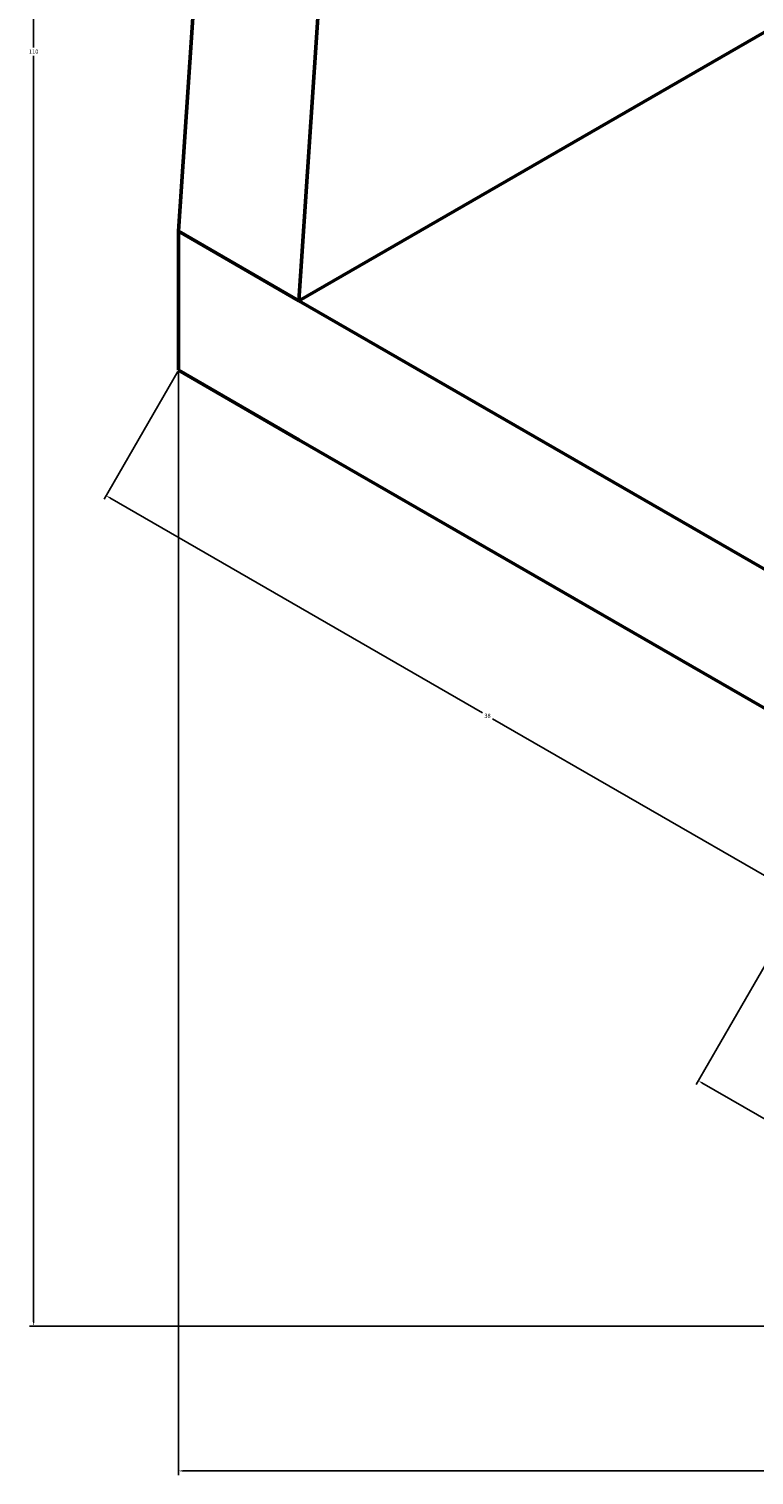
# Model space of a CAD drawing. Units: inches. Extents: x -23 to 69, y -27 to 96.
# Tile 1 of 10: x -23 to 8, y -27 to 35. Entities that reach past the tile are written whole.
import ezdxf

# ---------------------------------------------------------------- set-up
doc = ezdxf.new("R2010")
doc.units = ezdxf.units.IN
doc.header["$MEASUREMENT"] = 0
doc.layers.add('M-DIMS', color=2, linetype='Continuous', lineweight=18)
doc.layers.add('M-OUTL', color=7, linetype='Continuous', lineweight=50)
doc.styles.get("Standard").update_dxf_attribs({"font": 'arial.ttf'})
doc.dimstyles.get("Standard").update_dxf_attribs({"dimtxt": 0.18, "dimasz": 0.18, "dimexe": 0.18, "dimexo": 0.0625, "dimgap": 0.09, "dimtad": 0, "dimtih": 1, "dimtoh": 1, "dimdec": 4, "dimzin": 0, "dimdsep": 46, "dimtxsty": 'Standard', "dimcen": 0.09, "dimadec": 0, "dimazin": 0, "dimtfac": 1, "dimtdec": 4, "dimtofl": 0, "dimtmove": 0, "dimatfit": 3, "dimfxl": 1, "dimtolj": 1, "dimtzin": 0, "dimarcsym": 0})

# ---------------------------------------------------------------- blocks, each defined once
blk = doc.blocks.new('*D2')
at = {"layer": 'Defpoints', "color": 0, "transparency": 16777216}
for p in [(-16.638, 20.369), (-19.763, 14.956), (16.271, 1.369)]:
    blk.add_point(p, dxfattribs=at)
at = {"layer": 'M-DIMS', "color": 0, "lineweight": -2, "transparency": 16777216}
for p, q in [((-16.669, 20.315), (-19.853, 14.8)), ((-19.607, 14.866), (-3.527, 5.582)), ((12.99, -3.954), (-3.089, 5.33)), ((16.24, 1.315), (13.056, -4.2))]:
    blk.add_line(p, q, dxfattribs=at)
at = {"layer": 'M-DIMS', "color": 0, "transparency": 16777216}
for points in [[(-19.592, 14.892), (-19.622, 14.84), (-19.763, 14.956)], [(13.005, -3.928), (12.975, -3.98), (13.146, -4.044)]]:
    blk.add_solid(points, dxfattribs=at)
at = {"layer": 'M-DIMS', "color": 0, "transparency": 16777216, "insert": (-3.308, 5.456), "char_height": 0.18, "attachment_point": 5}
blk.add_mtext('\\A1;38', dxfattribs=at)
blk = doc.blocks.new('*D6')
at = {"layer": 'Defpoints', "color": 0, "transparency": 16777216}
for p in [(8.91, -4.881), (5.785, -10.294), (36.623, -20.881)]:
    blk.add_point(p, dxfattribs=at)
at = {"layer": 'M-DIMS', "color": 0, "lineweight": -2, "transparency": 16777216}
for p, q in [((8.879, -4.935), (5.695, -10.45)), ((5.941, -10.384), (19.423, -18.168)), ((33.342, -26.204), (19.859, -18.42)), ((36.592, -20.935), (33.408, -26.45))]:
    blk.add_line(p, q, dxfattribs=at)
at = {"layer": 'M-DIMS', "color": 0, "transparency": 16777216}
for points in [[(5.956, -10.358), (5.926, -10.41), (5.785, -10.294)], [(33.357, -26.178), (33.327, -26.23), (33.498, -26.294)]]:
    blk.add_solid(points, dxfattribs=at)
at = {"layer": 'M-DIMS', "color": 0, "transparency": 16777216, "insert": (19.641, -18.294), "char_height": 0.18, "attachment_point": 5}
blk.add_mtext('\\A1;32', dxfattribs=at)
blk = doc.blocks.new('*D13')
at = {"layer": 'Defpoints', "color": 0, "transparency": 16777216}
for p in [(15.838, 89.119), (-22.888, -20.881), (36.623, -20.881)]:
    blk.add_point(p, dxfattribs=at)
at = {"layer": 'M-DIMS', "color": 0, "lineweight": -2, "transparency": 16777216}
for p, q in [((15.776, 89.119), (-23.068, 89.119)), ((-22.888, 88.939), (-22.888, 34.301)), ((-22.888, -20.701), (-22.888, 33.937)), ((36.56, -20.881), (-23.068, -20.881))]:
    blk.add_line(p, q, dxfattribs=at)
at = {"layer": 'M-DIMS', "color": 0, "transparency": 16777216}
for points in [[(-22.918, 88.939), (-22.858, 88.939), (-22.888, 89.119)], [(-22.918, -20.701), (-22.858, -20.701), (-22.888, -20.881)]]:
    blk.add_solid(points, dxfattribs=at)
at = {"layer": 'M-DIMS', "color": 0, "transparency": 16777216, "insert": (-22.888, 34.119), "char_height": 0.18, "attachment_point": 5}
blk.add_mtext('\\A1;110', dxfattribs=at)
blk = doc.blocks.new('*D17')
at = {"layer": 'Defpoints', "color": 0, "transparency": 16777216}
for p in [(62.171, 27.869), (-16.638, 20.369), (62.171, -27.131)]:
    blk.add_point(p, dxfattribs=at)
at = {"layer": 'M-DIMS', "color": 0, "lineweight": -2, "transparency": 16777216}
for p, q in [((62.171, 27.806), (62.171, -27.311)), ((-16.638, 20.306), (-16.638, -27.311)), ((-16.458, -27.131), (22.391, -27.131)), ((61.991, -27.131), (23.142, -27.131))]:
    blk.add_line(p, q, dxfattribs=at)
at = {"layer": 'M-DIMS', "color": 0, "transparency": 16777216}
for points in [[(-16.458, -27.101), (-16.458, -27.161), (-16.638, -27.131)], [(61.991, -27.101), (61.991, -27.161), (62.171, -27.131)]]:
    blk.add_solid(points, dxfattribs=at)
at = {"layer": 'M-DIMS', "color": 0, "transparency": 16777216, "insert": (22.766, -27.131), "char_height": 0.18, "attachment_point": 5}
blk.add_mtext('\\A1;78.81', dxfattribs=at)

msp = doc.modelspace()

# ---------------------------------------------------------------- linework, layer by layer
at = {"layer": 'M-OUTL'}
for p, q in [((-13.6066, 72.1186), (-16.6377, 26.3686)), ((-8.4105, 69.1186), (-11.4416, 23.3686)), ((34.4578, 49.8686), (-11.4416, 23.3686)), ((-16.6377, 20.3686), (-16.6377, 26.3686)), ((-16.6377, 26.3686), (-11.4416, 23.3686)), ((-11.4416, 23.3686), (16.2712, 7.3686)), ((-11.4416, 17.3686), (-16.6377, 20.3686)), ((-11.4416, 17.3686), (16.2712, 1.3686))]:
    msp.add_line(p, q, dxfattribs=at)

# ---------------------------------------------------------------- dimensions: what is measured, and where the dimension line sits
at = {"layer": 'M-DIMS'}
for base, p1, p2, angle, picture, middle in [((-22.8877, -20.8814), (15.8382, 89.1186), (36.6228, -20.8814), 90, '*D13', (-22.8877, 34.1186)), ((-19.7627, 14.956), (16.2712, 1.3686), (-16.6377, 20.3686), 150, '*D2', (-3.3083, 5.456)), ((5.785, -10.294), (36.6228, -20.8814), (8.91, -4.8814), 150, '*D6', (19.6414, -18.294))]:
    dim = msp.add_linear_dim(base=base, p1=p1, p2=p2, angle=angle, dimstyle='Standard', override={"dimdec": 0, "dimlfac": 1, "dimrnd": 0, "dimzin": 0, "dimdsep": 46, "dimlunit": 2}, dxfattribs=at)
    dim.commit()
    dim.dimension.update_dxf_attribs({"geometry": picture, "text_midpoint": middle})
dim = msp.add_linear_dim(base=(62.1706, -27.1314), p1=(-16.6377, 20.3686), p2=(62.1706, 27.8686), dimstyle='Standard', override={"dimdec": 2, "dimlfac": 1, "dimrnd": 0, "dimzin": 0, "dimdsep": 46, "dimlunit": 2}, dxfattribs=at)
dim.commit()
dim.dimension.update_dxf_attribs({"geometry": '*D17', "text_midpoint": (22.7664, -27.1314)})

doc.saveas('drawing.dxf')
